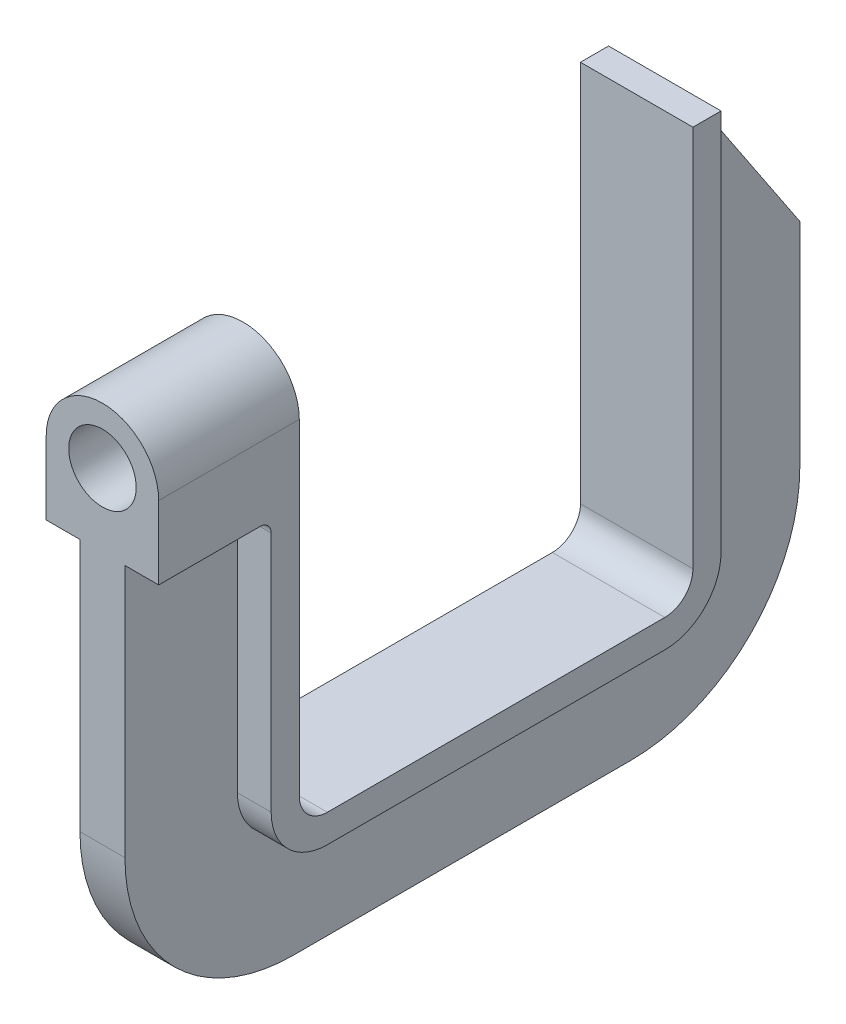
from build123d import *

# Parameters (mm, degrees)
C_FRAME_BODY_DEPTH  = 4
FRAME_RIM_DEPTH     = 10
SCREW_BOSS_DEPTH    = 25
SCREW_BORE_SKETCH_R = 6
SCREW_BORE_12_DEPTH = 43
EDGE_FILLETS_R2_R   = 2


with BuildPart() as part:
    # C-Frame Profile Sketch → C-Frame Body (new, symmetric)
    with BuildSketch(Plane(origin=(0, 0, 0), x_dir=(0, 0, -1), z_dir=(1, 0, 0))):
        with BuildLine():
            Line((0, 75), (0, 30))
            ThreePointArc((0, 30), (8.786796564, 8.786796564), (30, 0))
            Line((30, 0), (90, 0))
            ThreePointArc((90, 0), (111.213203436, 8.786796564), (120, 30))
            Line((120, 30), (120, 68))
            Line((120, 68), (100, 98))
            Line((100, 98), (95, 98))
            Line((95, 98), (95, 30))
            ThreePointArc((95, 30), (93.535533906, 26.464466094), (90, 25))
            Line((90, 25), (30, 25))
            ThreePointArc((30, 25), (26.464466094, 26.464466094), (25, 30))
            Line((25, 30), (25, 75))
            Line((25, 75), (0, 75))
        make_face()
    extrude(amount=C_FRAME_BODY_DEPTH, both=True)

    # Frame Rim Sketch → Frame Rim (add, symmetric)
    with BuildSketch(Plane(origin=(0, 0, 0), x_dir=(0, 0, -1), z_dir=(1, 0, 0))):
        with BuildLine():
            Line((25, 75), (20, 75))
            Line((20, 75), (20, 30))
            ThreePointArc((20, 30), (22.928932188, 22.928932188), (30, 20))
            Line((30, 20), (90, 20))
            ThreePointArc((90, 20), (97.071067812, 22.928932188), (100, 30))
            Line((100, 30), (100, 98))
            Line((100, 98), (95, 98))
            Line((95, 98), (95, 30))
            ThreePointArc((95, 30), (93.535533906, 26.464466094), (90, 25))
            Line((90, 25), (30, 25))
            ThreePointArc((30, 25), (26.464466094, 26.464466094), (25, 30))
            Line((25, 30), (25, 75))
        make_face()
    extrude(amount=FRAME_RIM_DEPTH, both=True)

    # Screw Boss Sketch → Screw Boss (add)
    with BuildSketch(Plane.XY):
        with BuildLine():
            Line((-10, 75), (10, 75))
            Line((10, 75), (10, 88))
            ThreePointArc((10, 88), (0, 98), (-10, 88))
            Line((-10, 88), (-10, 75))
        make_face()
    extrude(amount=-SCREW_BOSS_DEPTH)

    # Screw Bore Sketch → Screw Bore Ø12 (cut)
    with BuildSketch(Plane.XY):
        with Locations((0, 88)):
            Circle(SCREW_BORE_SKETCH_R)
    extrude(amount=-SCREW_BORE_12_DEPTH, mode=Mode.SUBTRACT)

    # Edge Fillets R2
    edge_fillets_r2_edges = [part.edges().sort_by_distance(p)[0] for p in [
        (7, 75, -20),
        (-7, 75, -20),
    ]]
    fillet(edge_fillets_r2_edges, radius=EDGE_FILLETS_R2_R)


solid = part.part
